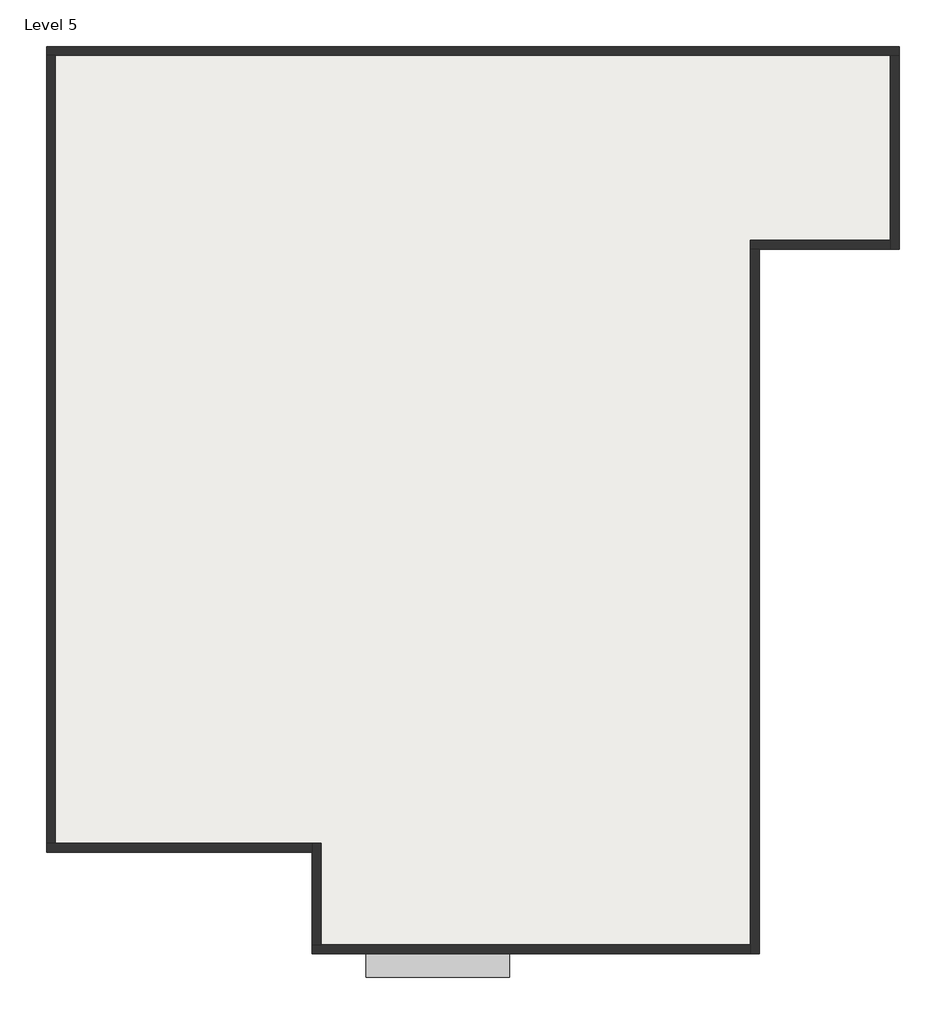
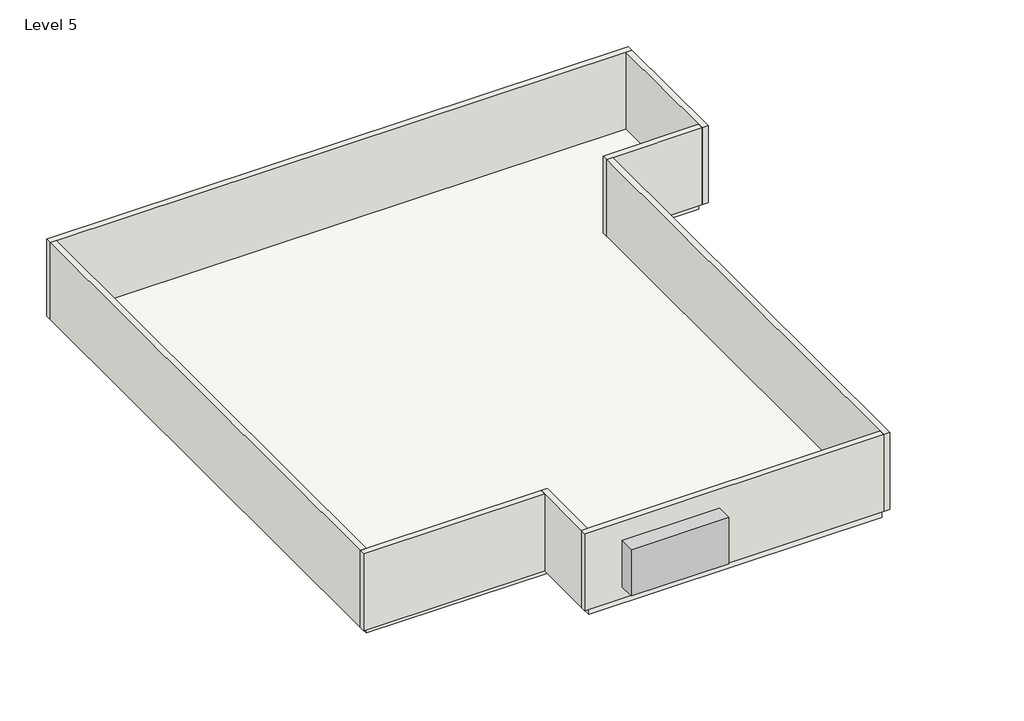
# One storey: 8 walls, 1 proxy, 1 roof.
"""IFC4 building model written with IfcOpenShell, lengths in millimetres."""

from ifc_helpers import new_model, si_unit, frame, origin, place, context, project, spatial, polyline, outline, extrude, faceted_brep, transform, mapped, element, save
from components import generic_models_3_generic_models_3_5aabad8c

model = new_model("IFC4")

# Units and contexts
model_context = context("Model", 3, world=origin())
ifc_project = project(units=[si_unit("LENGTHUNIT", "METRE", prefix="MILLI")], contexts=[model_context])

# Site, building, storey
site = spatial("IfcSite", under=ifc_project)
building = spatial("IfcBuilding", under=site)
storey = spatial("IfcBuildingStorey", under=building, Name="Level 5", Elevation=9601.2)

# Proxy
placement = place(None, origin())
generic_models_3_generic_models_3_shape = generic_models_3_generic_models_3_5aabad8c(model_context)
element("IfcBuildingElementProxy", 1, Name="Generic Models 3 : Generic Models 3", ObjectType="Generic Models 3 : Generic Models 3", at=placement, inside=storey, context=model_context, shape_type="MappedRepresentation", body=[
    mapped(generic_models_3_generic_models_3_shape, transform((0.0, 0.0, 0.0), x_axis=(1.0, 0.0, 0.0), y_axis=(0.0, 1.0, 0.0), z_axis=(0.0, 0.0, 1.0))),
])

# Roof
element("IfcRoof", 2, ObjectType="Generic - 12\"", at=placement, inside=storey, context=model_context, shape_type="SweptSolid", body=[
    extrude(outline(polyline([(-6132.0415084, 8043.8940003), (4535.9584916, 8043.8940003), (4535.9584916, 5681.6935985), (2745.2584916, 5681.6935985), (2745.2584916, -3360.7064015), (-2741.1415084, -3360.7064015), (-2741.1415084, -2014.5064015), (-6132.0415084, -2014.5064015), (-6132.0415084, 8043.8940003)])), frame((0.0, 0.0, 9448.8), z_axis=(0.0, 0.0, 1.0), x_axis=(1.0, 0.0, 0.0)), (0.0, 0.0, 1.0), 152.4),
])

# Walls
element("IfcWall", 3, ObjectType="WALL4.5\"", at=placement, inside=storey, context=model_context, shape_type="Brep", body=[
    faceted_brep([(-6246.3415084, 8043.8935985, 9601.2), (-6132.0415084, 8043.8935985, 9601.2), (4535.9584916, 8043.8935985, 9601.2), (4650.2584916, 8043.8935985, 9601.2), (4650.2584916, 8043.8935985, 11125.2), (4535.9584916, 8043.8935985, 11125.2), (-6132.0415084, 8043.8935985, 11125.2), (-6246.3415084, 8043.8935985, 11125.2), (-6246.3415084, 8158.1935985, 9601.2), (-6246.3415084, 8158.1935985, 11125.2), (4650.2584916, 8158.1935985, 11125.2), (4650.2584916, 8158.1935985, 9601.2)], [[[0, 1, 2, 3, 4, 5, 6, 7]], [[8, 9, 10, 11]], [[3, 2, 1, 0, 8, 11]], [[7, 6, 5, 4, 10, 9]], [[4, 3, 11, 10]], [[0, 7, 9, 8]]]),
])
element("IfcWall", 4, ObjectType="WALL4.5\"", at=placement, inside=storey, context=model_context, shape_type="Brep", body=[
    faceted_brep([(4535.9584916, 8043.8935985, 9601.2), (4535.9584916, 5681.6935985, 9601.2), (4535.9584916, 5567.3935985, 9601.2), (4535.9584916, 5567.3935985, 11125.2), (4535.9584916, 5681.6935985, 11125.2), (4535.9584916, 8043.8935985, 11125.2), (4650.2584916, 8043.8935985, 9601.2), (4650.2584916, 8043.8935985, 11125.2), (4650.2584916, 5567.3935985, 11125.2), (4650.2584916, 5567.3935985, 9601.2)], [[[0, 1, 2, 3, 4, 5]], [[6, 7, 8, 9]], [[2, 1, 0, 6, 9]], [[5, 4, 3, 8, 7]], [[0, 5, 7, 6]], [[3, 2, 9, 8]]]),
])
element("IfcWall", 5, ObjectType="WALL4.5\"", at=placement, inside=storey, context=model_context, shape_type="Brep", body=[
    faceted_brep([(4535.9584916, 5681.6935985, 9601.2), (2745.2584916, 5681.6935985, 9601.2), (2745.2584916, 5681.6935985, 11125.2), (4535.9584916, 5681.6935985, 11125.2), (4535.9584916, 5567.3935985, 9601.2), (4535.9584916, 5567.3935985, 11125.2), (2859.5584916, 5567.3935985, 11125.2), (2745.2584916, 5567.3935985, 11125.2), (2745.2584916, 5567.3935985, 9601.2), (2859.5584916, 5567.3935985, 9601.2)], [[[0, 1, 2, 3]], [[4, 5, 6, 7, 8, 9]], [[1, 0, 4, 9, 8]], [[3, 2, 7, 6, 5]], [[0, 3, 5, 4]], [[2, 1, 8, 7]]]),
])
element("IfcWall", 6, ObjectType="WALL4.5\"", at=placement, inside=storey, context=model_context, shape_type="Brep", body=[
    faceted_brep([(2745.2584916, 5567.3935985, 9601.2), (2745.2584916, -3309.9064015, 9601.2), (2745.2584916, -3424.2064015, 9601.2), (2745.2584916, -3424.2064015, 11125.2), (2745.2584916, -3309.9064015, 11125.2), (2745.2584916, 5567.3935985, 11125.2), (2859.5584916, 5567.3935985, 9601.2), (2859.5584916, 5567.3935985, 11125.2), (2859.5584916, -3424.2064015, 11125.2), (2859.5584916, -3424.2064015, 9601.2)], [[[0, 1, 2, 3, 4, 5]], [[6, 7, 8, 9]], [[2, 1, 0, 6, 9]], [[5, 4, 3, 8, 7]], [[0, 5, 7, 6]], [[3, 2, 9, 8]]]),
])
element("IfcWall", 7, ObjectType="WALL4.5\"", at=placement, inside=storey, context=model_context, shape_type="Brep", body=[
    faceted_brep([(2745.2584916, -3309.9064015, 9601.2), (-2741.1415084, -3309.9064015, 9601.2), (-2855.4415084, -3309.9064015, 9601.2), (-2855.4415084, -3309.9064015, 11125.2), (-2741.1415084, -3309.9064015, 11125.2), (2745.2584916, -3309.9064015, 11125.2), (2745.2584916, -3424.2064015, 9601.2), (2745.2584916, -3424.2064015, 11125.2), (-2855.4415084, -3424.2064015, 11125.2), (-2855.4415084, -3424.2064015, 9601.2)], [[[0, 1, 2, 3, 4, 5]], [[6, 7, 8, 9]], [[2, 1, 0, 6, 9]], [[5, 4, 3, 8, 7]], [[0, 5, 7, 6]], [[3, 2, 9, 8]]]),
])
element("IfcWall", 8, ObjectType="WALL4.5\"", at=placement, inside=storey, context=model_context, shape_type="Brep", body=[
    faceted_brep([(-2741.1415084, -3309.9064015, 9601.2), (-2741.1415084, -2014.5064015, 9601.2), (-2741.1415084, -2014.5064015, 11125.2), (-2741.1415084, -3309.9064015, 11125.2), (-2855.4415084, -3309.9064015, 9601.2), (-2855.4415084, -3309.9064015, 11125.2), (-2855.4415084, -2128.8064015, 11125.2), (-2855.4415084, -2014.5064015, 11125.2), (-2855.4415084, -2014.5064015, 9601.2), (-2855.4415084, -2128.8064015, 9601.2)], [[[0, 1, 2, 3]], [[4, 5, 6, 7, 8, 9]], [[1, 0, 4, 9, 8]], [[3, 2, 7, 6, 5]], [[0, 3, 5, 4]], [[2, 1, 8, 7]]]),
])
element("IfcWall", 9, ObjectType="WALL4.5\"", at=placement, inside=storey, context=model_context, shape_type="Brep", body=[
    faceted_brep([(-2855.4415084, -2014.5064015, 9601.2), (-6132.0415084, -2014.5064015, 9601.2), (-6246.3415084, -2014.5064015, 9601.2), (-6246.3415084, -2014.5064015, 11125.2), (-6132.0415084, -2014.5064015, 11125.2), (-2855.4415084, -2014.5064015, 11125.2), (-2855.4415084, -2128.8064015, 9601.2), (-2855.4415084, -2128.8064015, 11125.2), (-6246.3415084, -2128.8064015, 11125.2), (-6246.3415084, -2128.8064015, 9601.2)], [[[0, 1, 2, 3, 4, 5]], [[6, 7, 8, 9]], [[2, 1, 0, 6, 9]], [[5, 4, 3, 8, 7]], [[0, 5, 7, 6]], [[3, 2, 9, 8]]]),
])
element("IfcWall", 10, ObjectType="WALL4.5\"", at=placement, inside=storey, context=model_context, shape_type="SweptSolid", body=[
    extrude(outline(polyline([(-6132.0415084, 8043.8935985), (-6132.0415084, -2014.5064015), (-6246.3415084, -2014.5064015), (-6246.3415084, 8043.8935985), (-6132.0415084, 8043.8935985)])), frame((0.0, 0.0, 9601.2), z_axis=(0.0, 0.0, 1.0), x_axis=(1.0, 0.0, 0.0)), (0.0, 0.0, 1.0), 1524.0),
])

save(model, "model.ifc")

# Revit data of these elements
# Type "Generic - 12\""
#   Assembly Code = "B1020"
#   Layers, outside or top first: 0' - 6" no material (function 1)
# Type "WALL4.5\""
#   Assembly Code = "B2010"
#   Layers, outside or top first: 0' - 4 1/2" no material (function 1)
# Element 1 (IfcBuildingElementProxy, "Generic Models 3 : Generic Models 3")
#   Phase Created = New Construction
#   Materials on its faces: "Parking Stripe"
# Element 2 (IfcRoof, "Generic - 12\"")
#   built-in parameter 1001705 = 31.5 (stored number, unit not read)
#   built-in parameter 1001701 = -0.5 (stored number, unit not read)
#   built-in parameter 1001710 = 33615
#   Phase Created = New Construction
#   Materials on its faces: "Default Roof", "Wood - Stained"
# Elements 3, 4, 5, 6, 7, 8, 9, 10 (IfcWall, "WALL4.5\"")
#   Top Offset = 0' - 0"
#   Base Offset = 0' - 0"
#   Unconnected Height = 5' - 0"
#   wall height = 5' - 0"
#   Phase Created = New Construction
#   Base Constraint = Level 5
#   Materials on its faces: "Default Wall"
# Materials
#   "Parking Stripe": class "Paint", colour RGB 250 250 91, transparency 0, Cost = 0
#   "Default Roof": colour RGB 88 101 114, transparency 0, Cost = 0
#   "Wood - Stained": class "Wood", colour RGB 224 178 126, transparency 0, Cost = 0
#   "Default Wall": colour RGB 128 128 128, transparency 0, Cost = 0
